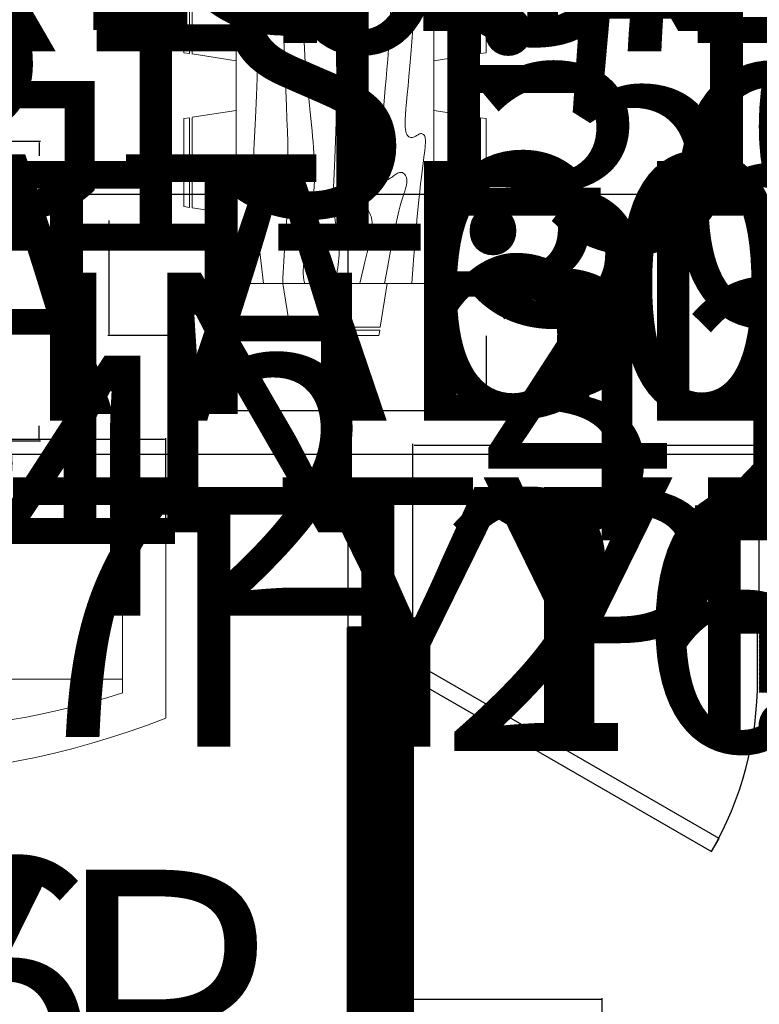
# Model space of a CAD drawing. Units: inches. Extents: x 1173 to 2157, y 515 to 1129.
# Tile 5 of 13: x 1475 to 1578, y 743 to 880. Entities that reach past the tile are written whole.
import ezdxf

# ---------------------------------------------------------------- set-up
doc = ezdxf.new("R2010")
doc.units = ezdxf.units.IN
doc.header["$MEASUREMENT"] = 0
for name, color, linetype, lineweight in [('A-ANNO-DIMS', 2, 'Continuous', 18), ('A-DOOR', 3, 'Continuous', 25), ('A-FURN', 8, 'Continuous', 18), ('A-WALL', 7, 'Continuous', 50)]:
    doc.layers.add(name, color=color, linetype=linetype, lineweight=lineweight)
doc.layers.add('A-WALL-PATT', color=22, linetype='Continuous', lineweight=13, true_color=0xca4b0c)
doc.styles.get("Standard").update_dxf_attribs({"font": 'arial.ttf'})
doc.dimstyles.get("Standard").update_dxf_attribs({"dimtxt": 36, "dimasz": 0.18, "dimexe": 0.18, "dimexo": 0.0625, "dimgap": 0.09, "dimtad": 0, "dimtih": 1, "dimtoh": 1, "dimdec": 0, "dimrnd": 72, "dimzin": 0, "dimdsep": 46, "dimlunit": 3, "dimtxsty": 'Standard', "dimcen": 2, "dimadec": 0, "dimazin": 0, "dimtfac": 1, "dimtdec": 0, "dimtofl": 0, "dimtmove": 0, "dimatfit": 3, "dimfxl": 1, "dimtolj": 1, "dimtzin": 0, "dimarcsym": 0})

# ---------------------------------------------------------------- blocks, each defined once
blk = doc.blocks.new('*U4')
for p, q in [((0, 0), (0, 6)), ((40, 0), (40, 6))]:
    blk.add_line(p, q)
blk.add_lwpolyline([(0, 0), (34.64, -20), (35.52, -18.48), (0.87, 1.52)], close=True)
blk.add_arc((0, 0), 40, 330, 0)
blk = doc.blocks.new('Dining Set - 36 x 72 in.')
for p, q in [((-22, 27.5), (-22.1562, 26.50042)), ((-22, 27.5), (-6, 27.5)), ((-5.8437, 26.49966), (-6, 27.5)), ((6, 27.5), (5.8438, 26.50042)), ((6, 27.5), (22, 27.5)), ((22.1563, 26.49966), (22, 27.5)), ((-22.2343, 26.00059), (-23.4847, 17.99762)), ((-22.2304, 26), (-5.7608, 26)), ((-5.8416, 26.5), (-22.1534, 26.5)), ((-4.5152, 17.99762), (-5.7655, 25.99926)), ((5.7657, 26.00059), (4.5153, 17.99762)), ((5.7696, 26), (22.2392, 26)), ((22.1584, 26.5), (5.8466, 26.5)), ((23.4848, 17.99762), (22.2345, 25.99926)), ((36, 18), (-36, 18)), ((-36, 18), (-36, -18)), ((36, -18), (36, 18)), ((-44.0006, 8.23428), (-35.9976, 9.48474)), ((44.0006, 8.23428), (35.9976, 9.48474)), ((-45.5, 8), (-44.5004, 8.15617)), ((-45.5, 8), (-45.5, -8)), ((-44.5, -8.15843), (-44.5, 8.15338)), ((-44, 8.23041), (-44, -8.23915)), ((44, 8.23041), (44, -8.23915)), ((44.5, -8.15843), (44.5, 8.15338)), ((45.5, 8), (44.5005, 8.15617)), ((45.5, 8), (45.5, -8)), ((-44.4997, -8.15631), (-45.5, -8)), ((-35.9976, -9.48476), (-43.9993, -8.2345)), ((35.9976, -9.48476), (43.9993, -8.2345)), ((44.4997, -8.15631), (45.5, -8)), ((-36, -18), (36, -18)), ((-22.2343, -26.0006), (-23.4847, -17.99762)), ((-4.5152, -17.99762), (-5.7655, -25.99928)), ((5.7657, -26.0006), (4.5153, -17.99762)), ((23.4848, -17.99762), (22.2345, -25.99928)), ((-22.2304, -26), (-5.7608, -26)), ((-22, -27.5), (-22.1562, -26.50044)), ((-5.8416, -26.5), (-22.1534, -26.5)), ((-5.8437, -26.49967), (-6, -27.5)), ((5.7696, -26), (22.2392, -26)), ((6, -27.5), (5.8438, -26.50044)), ((22.1584, -26.5), (5.8466, -26.5)), ((22.1563, -26.49967), (22, -27.5)), ((-22, -27.5), (-6, -27.5)), ((6, -27.5), (22, -27.5))]:
    blk.add_line(p, q)
for points in [[(-36, 15), (-31.1772, 14.97754), (-26.8079, 14.91406), (-22.8538, 14.81543), (-19.276, 14.6875), (-16.0362, 14.53613), (-13.0957, 14.36718), (-10.4159, 14.18652), (-7.9583, 14), (-5.6904, 13.81315), (-3.6035, 13.63021), (-1.6954, 13.45508), (0.0365, 13.29166), (1.5945, 13.14388), (2.9811, 13.01562), (4.1988, 12.9108), (5.25, 12.83333), (6.1393, 12.78613), (6.8802, 12.76823), (7.4883, 12.77767), (7.9792, 12.8125), (8.3685, 12.87077), (8.6719, 12.95052), (8.9049, 13.0498), (9.0833, 13.16666), (9.2205, 13.29899), (9.3216, 13.44401), (9.3895, 13.59879), (9.4271, 13.76041), (9.4373, 13.92594), (9.4232, 14.09245), (9.3875, 14.257), (9.3333, 14.41666), (9.2638, 14.56917), (9.1836, 14.71484), (9.0975, 14.85465), (9.0104, 14.98958), (8.9272, 15.1206), (8.8529, 15.2487), (8.7922, 15.37483), (8.75, 15.5), (8.7305, 15.62467), (8.7344, 15.74739), (8.7617, 15.86621), (8.8125, 15.97916), (8.8867, 16.08431), (8.9844, 16.17968), (9.1055, 16.26334), (9.25, 16.33333), (9.4189, 16.38802), (9.6172, 16.42708), (9.8506, 16.45052), (10.125, 16.45833), (10.4463, 16.45052), (10.8203, 16.42708), (11.2529, 16.38802), (11.75, 16.33333), (12.3184, 16.26318), (12.9694, 16.17838), (13.7151, 16.07991), (14.5677, 15.96875), (15.5395, 15.84586), (16.6426, 15.71224), (17.8893, 15.56884), (19.2917, 15.41666), (20.859, 15.25667), (22.5879, 15.08984), (24.4721, 14.91715), (26.5052, 14.73958), (28.6809, 14.5581), (30.9929, 14.3737), (33.4347, 14.18733), (36, 14)], [(-36, 10), (-28.9766, 10.14274), (-23.1725, 10.20442), (-18.4241, 10.19775), (-14.5677, 10.13541), (-11.4399, 10.03011), (-8.877, 9.89453), (-6.7154, 9.74137), (-4.7917, 9.58333), (-2.9698, 9.43082), (-1.2246, 9.28515), (0.4415, 9.14534), (2.026, 9.01041), (3.5266, 8.87939), (4.9408, 8.7513), (6.266, 8.62516), (7.5, 8.5), (8.6411, 8.37549), (9.6914, 8.2539), (10.6538, 8.13818), (11.5312, 8.03125), (12.3267, 7.93603), (13.043, 7.85547), (13.6831, 7.79248), (14.25, 7.75), (14.7471, 7.7303), (15.1797, 7.73307), (15.5537, 7.75732), (15.875, 7.80208), (16.1494, 7.86637), (16.3828, 7.94922), (16.5811, 8.04964), (16.75, 8.16666), (16.8944, 8.29915), (17.0143, 8.44531), (17.1089, 8.60319), (17.1771, 8.77083), (17.218, 8.94629), (17.2305, 9.1276), (17.2137, 9.31282), (17.1667, 9.5), (17.0895, 9.6875), (16.987, 9.875), (16.8649, 10.0625), (16.7292, 10.25), (16.5856, 10.4375), (16.4401, 10.625), (16.2985, 10.8125), (16.1667, 11), (16.05, 11.18733), (15.9518, 11.3737), (15.8752, 11.5581), (15.8229, 11.73958), (15.798, 11.91715), (15.8034, 12.08984), (15.842, 12.25667), (15.9167, 12.41666), (16.0295, 12.56836), (16.1784, 12.70833), (16.3605, 12.83268), (16.5729, 12.9375), (16.8127, 13.01888), (17.0768, 13.07291), (17.3625, 13.0957), (17.6667, 13.08333), (17.9894, 13.03312), (18.3418, 12.94726), (18.7382, 12.82918), (19.1927, 12.68229), (19.7195, 12.51001), (20.3327, 12.31575), (21.0465, 12.10294), (21.875, 11.875), (22.8357, 11.63354), (23.959, 11.37304), (25.2786, 11.08618), (26.8282, 10.76562), (28.6414, 10.40405), (30.752, 9.99414), (33.1936, 9.52856), (36, 9)], [(-36, 5.5), (-30.7157, 5.3348), (-26.069, 5.20963), (-21.9946, 5.11767), (-18.4271, 5.05208), (-15.3009, 5.00602), (-12.5508, 4.97265), (-10.1112, 4.94515), (-7.9167, 4.91666), (-5.909, 4.88167), (-4.0586, 4.83984), (-2.3429, 4.79215), (-0.7396, 4.73958), (0.7739, 4.6831), (2.22, 4.6237), (3.6213, 4.56233), (5, 4.5), (6.373, 4.43782), (7.7344, 4.3776), (9.0723, 4.32129), (10.375, 4.27083), (11.6309, 4.22819), (12.8281, 4.19531), (13.9551, 4.17415), (15, 4.16666), (15.954, 4.17448), (16.819, 4.19791), (17.6001, 4.23698), (18.3021, 4.29166), (18.9299, 4.36198), (19.4883, 4.44791), (19.9823, 4.54948), (20.4167, 4.66666), (20.7969, 4.79899), (21.1302, 4.94401), (21.4245, 5.09879), (21.6875, 5.26041), (21.9271, 5.42594), (22.1511, 5.59245), (22.3672, 5.757), (22.5834, 5.91666), (22.8065, 6.06868), (23.0404, 6.21093), (23.2879, 6.34147), (23.5521, 6.45833), (23.8358, 6.55957), (24.142, 6.64323), (24.4735, 6.70735), (24.8334, 6.75), (25.2235, 6.76969), (25.642, 6.76692), (26.0858, 6.74267), (26.5521, 6.69791), (27.0379, 6.63362), (27.5404, 6.55078), (28.0565, 6.45036), (28.5834, 6.33333), (29.1242, 6.19987), (29.7071, 6.04687), (30.3661, 5.87044), (31.1354, 5.66666), (32.0493, 5.43164), (33.142, 5.16146), (34.4475, 4.85221), (36, 4.5)], [(-36, -1), (-30.7915, -0.6591), (-26.0195, -0.38216), (-21.6519, -0.16284), (-17.6563, 0.00521), (-14.0005, 0.12833), (-10.6523, 0.21289), (-7.5796, 0.26522), (-4.75, 0.29166), (-2.134, 0.29793), (0.2878, 0.28711), (2.5317, 0.26163), (4.6146, 0.22396), (6.5529, 0.17651), (8.3633, 0.12174), (10.0623, 0.06209), (11.6667, 0), (13.1899, -0.06201), (14.6341, -0.1211), (15.9982, -0.17432), (17.2813, -0.21875), (18.4823, -0.25147), (19.6003, -0.26953), (20.6343, -0.27002), (21.5834, -0.25), (22.4481, -0.20768), (23.2357, -0.14584), (23.9549, -0.06836), (24.6146, 0.02083), (25.2235, 0.11784), (25.7904, 0.21875), (26.3241, 0.31966), (26.8334, 0.41666), (27.3265, 0.50618), (27.8099, 0.58593), (28.2894, 0.65397), (28.7709, 0.70833), (29.2601, 0.74707), (29.763, 0.76823), (30.2855, 0.76985), (30.8334, 0.75), (31.4088, 0.70784), (31.9994, 0.64713), (32.589, 0.57275), (33.1615, 0.48958), (33.7008, 0.4025), (34.1908, 0.3164), (34.6153, 0.23616), (34.9584, 0.16666), (35.2099, 0.11165), (35.3848, 0.07031), (35.504, 0.04069), (35.5886, 0.02083), (35.6594, 0.00879), (35.7377, 0.0026), (35.8442, 0.00032), (36, 0)], [(-36, -6.5), (-27.1843, -6.31267), (-20.084, -6.1263), (-14.469, -5.9419), (-10.1094, -5.76042), (-6.7752, -5.58285), (-4.2363, -5.41016), (-2.2629, -5.24333), (-0.625, -5.08334), (0.8708, -4.93099), (2.2715, -4.78646), (3.5872, -4.64974), (4.8281, -4.52084), (6.0046, -4.39974), (7.127, -4.28646), (8.2053, -4.18099), (9.25, -4.08334), (10.2705, -3.99382), (11.2734, -3.91407), (12.2647, -3.84603), (13.25, -3.79167), (14.2354, -3.75293), (15.2266, -3.73177), (16.2295, -3.73015), (17.25, -3.75), (18.2912, -3.79248), (19.3451, -3.85547), (20.4009, -3.93604), (21.4479, -4.03125), (22.4754, -4.13819), (23.4727, -4.25391), (24.4289, -4.37549), (25.3334, -4.5), (26.1785, -4.62492), (26.9694, -4.74935), (27.7145, -4.87281), (28.4219, -4.99479), (29.1, -5.11483), (29.7572, -5.23242), (30.4016, -5.34709), (31.0417, -5.45834), (31.6837, -5.56437), (32.3262, -5.65821), (32.9658, -5.73153), (33.599, -5.77604), (34.2224, -5.78345), (34.8327, -5.74545), (35.4264, -5.65373), (36, -5.5)], [(-36, -10), (-26.4022, -9.81299), (-18.4675, -9.62891), (-11.9839, -9.45069), (-6.7396, -9.28125), (-2.5226, -9.12354), (0.8789, -8.98047), (3.6769, -8.85498), (6.0833, -8.75), (8.2767, -8.66765), (10.3021, -8.60677), (12.1712, -8.56543), (13.8958, -8.54167), (15.4876, -8.53353), (16.9583, -8.53907), (18.3197, -8.55632), (19.5834, -8.58334), (20.7616, -8.61841), (21.8685, -8.66081), (22.9188, -8.71004), (23.9271, -8.76563), (24.9081, -8.82707), (25.8763, -8.89388), (26.8465, -8.96558), (27.8334, -9.04167), (28.8474, -9.12118), (29.8828, -9.20117), (30.93, -9.27824), (31.9792, -9.34896), (33.0205, -9.40991), (34.0443, -9.45768), (35.0407, -9.48885), (36, -9.5)], [(-36, -14.5), (-30.0881, -14.33513), (-25.0332, -14.21224), (-20.7312, -14.12647), (-17.0781, -14.07292), (-13.97, -14.04671), (-11.3027, -14.04297), (-8.9724, -14.05681), (-6.875, -14.08334), (-4.9224, -14.11833), (-3.0905, -14.16016), (-1.3709, -14.20785), (0.2448, -14.26042), (1.7647, -14.3169), (3.1973, -14.3763), (4.5507, -14.43767), (5.8333, -14.5), (7.0554, -14.5621), (8.235, -14.62175), (9.3922, -14.67652), (10.5469, -14.72396), (11.7192, -14.76164), (12.929, -14.78711), (14.1965, -14.79794), (15.5417, -14.79167), (16.9933, -14.76424), (18.6152, -14.70508), (20.4804, -14.60197), (22.6615, -14.44271), (25.2312, -14.21509), (28.2624, -13.9069), (31.8277, -13.50594), (36, -13)]]:
    blk.add_lwpolyline(points)
blk = doc.blocks.new('Sofa - Roundback 7 ft.')
for p, q in [((-12.00002, -32.4421), (-12.00003, -6.5971)), ((11.99997, -32.4421), (11.99998, -6.5971)), ((-36.000027, -34), (-36.000027, -11.4696)), ((35.99998, -34), (35.99998, -11.4696)), ((-35.999844, -13.3819), (35.9998, -13.3819)), ((-36.000027, -32.4421), (35.99998, -32.4421))]:
    blk.add_line(p, q)
for points in [[(-36.000027, -34), (-42.000027, -34), (-42.000027, -8)], [(41.99998, -8), (41.99998, -34), (35.99998, -34)]]:
    blk.add_lwpolyline(points)
for centre, radius, start, end in [((0, -114.25), 114.25, 68.43141, 111.5686), ((-0.00001, -127.1968), 121.1968, 72.72033, 107.2797)]:
    blk.add_arc(centre, radius, start, end)
blk = doc.blocks.new('*D26')
at = {"layer": 'A-ANNO-DIMS', "color": 0, "lineweight": -2, "transparency": 16777216}
for p, q in [((1577.15, 654.34), (1577.15, 661.66)), ((1577.33, 661.48), (1624.97, 661.48)), ((1625.15, 654.34), (1625.15, 661.66)), ((1625.15, 661.48), (1625.33, 661.48))]:
    blk.add_line(p, q, dxfattribs=at)
at = {"layer": 'A-ANNO-DIMS', "color": 0, "transparency": 16777216}
for points in [[(1577.33, 661.51), (1577.33, 661.45), (1577.15, 661.48)], [(1624.97, 661.51), (1624.97, 661.45), (1625.15, 661.48)]]:
    blk.add_solid(points, dxfattribs=at)
at = {"layer": 'Defpoints', "color": 0, "transparency": 16777216}
for p in [(1625.15, 661.48), (1577.15, 654.28), (1625.15, 654.28)]:
    blk.add_point(p, dxfattribs=at)
at = {"layer": 'A-ANNO-DIMS', "color": 0, "transparency": 16777216, "insert": (1831.09, 661.48), "char_height": 36, "attachment_point": 5}
blk.add_mtext('\\A1;WINDOW 48 TYP.', dxfattribs=at)
blk = doc.blocks.new('*D30')
at = {"layer": 'A-ANNO-DIMS', "color": 0, "lineweight": -2, "transparency": 16777216}
for p, q in [((1555.97, 736.03), (1563.78, 736.03)), ((1563.6, 735.85), (1563.6, 729.12)), ((1563.6, 684.97), (1563.6, 691.71)), ((1555.97, 684.79), (1563.78, 684.79))]:
    blk.add_line(p, q, dxfattribs=at)
at = {"layer": 'A-ANNO-DIMS', "color": 0, "transparency": 16777216}
for points in [[(1563.57, 735.85), (1563.63, 735.85), (1563.6, 736.03)], [(1563.57, 684.97), (1563.63, 684.97), (1563.6, 684.79)]]:
    blk.add_solid(points, dxfattribs=at)
at = {"layer": 'Defpoints', "color": 0, "transparency": 16777216}
for p in [(1555.91, 736.03), (1563.6, 736.03), (1555.91, 684.79)]:
    blk.add_point(p, dxfattribs=at)
at = {"layer": 'A-ANNO-DIMS', "color": 0, "transparency": 16777216, "insert": (1563.6, 710.41), "char_height": 36, "attachment_point": 5}
blk.add_mtext('\\A1;DESK 51 TYP.', dxfattribs=at)
blk = doc.blocks.new('*D31')
at = {"layer": 'A-ANNO-DIMS', "color": 0, "lineweight": -2, "transparency": 16777216}
for p, q in [((1529.44, 743.72), (1529.26, 743.72)), ((1529.44, 736.09), (1529.44, 743.9)), ((1555.73, 743.72), (1529.62, 743.72)), ((1555.91, 736.09), (1555.91, 743.9))]:
    blk.add_line(p, q, dxfattribs=at)
at = {"layer": 'A-ANNO-DIMS', "color": 0, "transparency": 16777216}
for points in [[(1529.62, 743.75), (1529.62, 743.69), (1529.44, 743.72)], [(1555.73, 743.75), (1555.73, 743.69), (1555.91, 743.72)]]:
    blk.add_solid(points, dxfattribs=at)
at = {"layer": 'Defpoints', "color": 0, "transparency": 16777216}
for p in [(1529.44, 743.72), (1529.44, 736.03), (1555.91, 736.03)]:
    blk.add_point(p, dxfattribs=at)
at = {"layer": 'A-ANNO-DIMS', "color": 0, "transparency": 16777216, "insert": (1441.24, 743.72), "char_height": 36, "attachment_point": 5}
blk.add_mtext('\\A1;26 TYP.', dxfattribs=at)
blk = doc.blocks.new('*D36')
at = {"layer": 'A-ANNO-DIMS', "color": 0, "lineweight": -2, "transparency": 16777216}
for p, q in [((1497.87, 905.02), (1487.37, 905.02)), ((1487.55, 904.84), (1487.55, 889.09)), ((1487.55, 835.93), (1487.55, 851.68)), ((1497.87, 835.75), (1487.37, 835.75))]:
    blk.add_line(p, q, dxfattribs=at)
at = {"layer": 'A-ANNO-DIMS', "color": 0, "transparency": 16777216}
for points in [[(1487.52, 904.84), (1487.58, 904.84), (1487.55, 905.02)], [(1487.52, 835.93), (1487.58, 835.93), (1487.55, 835.75)]]:
    blk.add_solid(points, dxfattribs=at)
at = {"layer": 'Defpoints', "color": 0, "transparency": 16777216}
for p in [(1497.94, 905.02), (1487.55, 835.75), (1497.94, 835.75)]:
    blk.add_point(p, dxfattribs=at)
at = {"layer": 'A-ANNO-DIMS', "color": 0, "transparency": 16777216, "insert": (1487.55, 870.38), "char_height": 36, "attachment_point": 5}
blk.add_mtext('\\A1;DINING SET 69', dxfattribs=at)
blk = doc.blocks.new('*D37')
at = {"layer": 'A-ANNO-DIMS', "color": 0, "lineweight": -2, "transparency": 16777216}
for p, q in [((1497.94, 835.69), (1497.94, 825.18)), ((1539.8, 835.69), (1539.8, 825.18)), ((1498.12, 825.36), (1539.62, 825.36)), ((1539.8, 825.36), (1539.98, 825.36))]:
    blk.add_line(p, q, dxfattribs=at)
at = {"layer": 'A-ANNO-DIMS', "color": 0, "transparency": 16777216}
for points in [[(1498.12, 825.39), (1498.12, 825.33), (1497.94, 825.36)], [(1539.62, 825.39), (1539.62, 825.33), (1539.8, 825.36)]]:
    blk.add_solid(points, dxfattribs=at)
at = {"layer": 'Defpoints', "color": 0, "transparency": 16777216}
for p in [(1497.94, 835.75), (1539.8, 835.75), (1539.8, 825.36)]:
    blk.add_point(p, dxfattribs=at)
at = {"layer": 'A-ANNO-DIMS', "color": 0, "transparency": 16777216, "insert": (1566.4, 825.36), "char_height": 36, "attachment_point": 5}
blk.add_mtext('\\A1;42', dxfattribs=at)
blk = doc.blocks.new('*D38')
at = {"layer": 'A-ANNO-DIMS', "color": 0, "lineweight": -2, "transparency": 16777216}
for p, q in [((1471.69, 862.7), (1478.04, 862.7)), ((1477.86, 862.52), (1477.86, 860.65)), ((1477.86, 821.35), (1477.86, 823.22)), ((1471.69, 821.17), (1478.04, 821.17))]:
    blk.add_line(p, q, dxfattribs=at)
at = {"layer": 'A-ANNO-DIMS', "color": 0, "transparency": 16777216}
for points in [[(1477.83, 862.52), (1477.89, 862.52), (1477.86, 862.7)], [(1477.83, 821.35), (1477.89, 821.35), (1477.86, 821.17)]]:
    blk.add_solid(points, dxfattribs=at)
at = {"layer": 'Defpoints', "color": 0, "transparency": 16777216}
for p in [(1471.63, 862.7), (1477.86, 862.7), (1471.63, 821.17)]:
    blk.add_point(p, dxfattribs=at)
at = {"layer": 'A-ANNO-DIMS', "color": 0, "transparency": 16777216, "insert": (1477.86, 841.93), "char_height": 36, "attachment_point": 5}
blk.add_mtext('\\A1;COFFEE TABLE 42', dxfattribs=at)
blk = doc.blocks.new('*D39')
at = {"layer": 'A-ANNO-DIMS', "color": 0, "lineweight": -2, "transparency": 16777216}
for p, q in [((1430.11, 821.11), (1430.11, 814.76)), ((1471.63, 821.11), (1471.63, 814.76)), ((1430.29, 814.94), (1471.45, 814.94)), ((1471.63, 814.94), (1471.81, 814.94))]:
    blk.add_line(p, q, dxfattribs=at)
at = {"layer": 'A-ANNO-DIMS', "color": 0, "transparency": 16777216}
for points in [[(1430.29, 814.97), (1430.29, 814.91), (1430.11, 814.94)], [(1471.45, 814.97), (1471.45, 814.91), (1471.63, 814.94)]]:
    blk.add_solid(points, dxfattribs=at)
at = {"layer": 'Defpoints', "color": 0, "transparency": 16777216}
for p in [(1430.11, 821.17), (1471.63, 821.17), (1471.63, 814.94)]:
    blk.add_point(p, dxfattribs=at)
at = {"layer": 'A-ANNO-DIMS', "color": 0, "transparency": 16777216, "insert": (1498.22, 814.94), "char_height": 36, "attachment_point": 5}
blk.add_mtext('\\A1;42', dxfattribs=at)
blk = doc.blocks.new('*D40')
at = {"layer": 'A-ANNO-DIMS', "color": 0, "lineweight": -2, "transparency": 16777216}
for p, q in [((1422.73, 872.86), (1431.84, 872.86)), ((1431.66, 872.68), (1431.66, 861.58)), ((1431.66, 813.04), (1431.66, 824.15)), ((1422.73, 812.86), (1431.84, 812.86))]:
    blk.add_line(p, q, dxfattribs=at)
at = {"layer": 'A-ANNO-DIMS', "color": 0, "transparency": 16777216}
for points in [[(1431.63, 872.68), (1431.69, 872.68), (1431.66, 872.86)], [(1431.63, 813.04), (1431.69, 813.04), (1431.66, 812.86)]]:
    blk.add_solid(points, dxfattribs=at)
at = {"layer": 'Defpoints', "color": 0, "transparency": 16777216}
for p in [(1422.66, 872.86), (1431.66, 872.86), (1422.66, 812.86)]:
    blk.add_point(p, dxfattribs=at)
at = {"layer": 'A-ANNO-DIMS', "color": 0, "transparency": 16777216, "insert": (1431.66, 842.86), "char_height": 36, "attachment_point": 5}
blk.add_mtext('\\A1;LOVESEAT 60', dxfattribs=at)
blk = doc.blocks.new('*D42')
at = {"layer": 'A-ANNO-DIMS', "color": 0, "lineweight": -2, "transparency": 16777216}
for p, q in [((1411.43, 808.8), (1411.43, 821.52)), ((1495.43, 808.8), (1495.43, 821.52)), ((1411.43, 821.34), (1411.25, 821.34)), ((1495.25, 821.34), (1411.61, 821.34))]:
    blk.add_line(p, q, dxfattribs=at)
at = {"layer": 'A-ANNO-DIMS', "color": 0, "transparency": 16777216}
for points in [[(1411.61, 821.37), (1411.61, 821.31), (1411.43, 821.34)], [(1495.25, 821.37), (1495.25, 821.31), (1495.43, 821.34)]]:
    blk.add_solid(points, dxfattribs=at)
at = {"layer": 'Defpoints', "color": 0, "transparency": 16777216}
for p in [(1411.43, 821.34), (1411.43, 808.74), (1495.43, 808.74)]:
    blk.add_point(p, dxfattribs=at)
at = {"layer": 'A-ANNO-DIMS', "color": 0, "transparency": 16777216, "insert": (1310.09, 821.34), "char_height": 36, "attachment_point": 5}
blk.add_mtext('\\A1;SOFA 84', dxfattribs=at)
blk = doc.blocks.new('*D46')
at = {"layer": 'A-ANNO-DIMS', "color": 0, "lineweight": -2, "transparency": 16777216}
for p, q in [((1646.37, 911.98), (1645.86, 896.32)), ((1648.72, 912.09), (1646.2, 912.17)), ((1645.85, 895.96), (1645.67, 895.96)), ((1648.2, 896.07), (1645.68, 896.15)), ((1645.86, 896.14), (1645.85, 895.96))]:
    blk.add_line(p, q, dxfattribs=at)
at = {"layer": 'A-ANNO-DIMS', "color": 0, "transparency": 16777216}
for points in [[(1646.34, 911.99), (1646.4, 911.98), (1646.38, 912.16)], [(1645.83, 896.32), (1645.89, 896.32), (1645.86, 896.14)]]:
    blk.add_solid(points, dxfattribs=at)
at = {"layer": 'Defpoints', "color": 0, "transparency": 16777216}
for p in [(1648.78, 912.09), (1645.86, 896.14), (1648.26, 896.06)]:
    blk.add_point(p, dxfattribs=at)
at = {"layer": 'A-ANNO-DIMS', "color": 0, "transparency": 16777216, "insert": (1538.16, 895.96), "char_height": 36, "attachment_point": 5}
blk.add_mtext('\\A1;BASIN 16', dxfattribs=at)
blk = doc.blocks.new('*D48')
at = {"layer": 'A-ANNO-DIMS', "color": 0, "lineweight": -2, "transparency": 16777216}
for p, q in [((1592.53, 826.46), (1592.35, 826.47)), ((1592.38, 821.85), (1592.54, 826.64)), ((1623.53, 825.46), (1592.71, 826.46)), ((1623.56, 820.84), (1623.71, 825.64))]:
    blk.add_line(p, q, dxfattribs=at)
at = {"layer": 'A-ANNO-DIMS', "color": 0, "transparency": 16777216}
for points in [[(1592.71, 826.49), (1592.71, 826.43), (1592.53, 826.46)], [(1623.53, 825.49), (1623.53, 825.43), (1623.71, 825.46)]]:
    blk.add_solid(points, dxfattribs=at)
at = {"layer": 'Defpoints', "color": 0, "transparency": 16777216}
for p in [(1592.53, 826.46), (1592.38, 821.79), (1623.56, 820.78)]:
    blk.add_point(p, dxfattribs=at)
at = {"layer": 'A-ANNO-DIMS', "color": 0, "transparency": 16777216, "insert": (1488.3, 826.47), "char_height": 36, "attachment_point": 5}
blk.add_mtext('\\A1;BASIN 31', dxfattribs=at)
blk = doc.blocks.new('*D49')
at = {"layer": 'A-ANNO-DIMS', "color": 0, "lineweight": -2, "transparency": 16777216}
for p, q in [((1587.7, 821.76), (1586.89, 796.55)), ((1592.32, 821.79), (1587.52, 821.94)), ((1586.87, 796.19), (1586.69, 796.19)), ((1591.49, 796.22), (1586.7, 796.37)), ((1586.88, 796.37), (1586.87, 796.19))]:
    blk.add_line(p, q, dxfattribs=at)
at = {"layer": 'A-ANNO-DIMS', "color": 0, "transparency": 16777216}
for points in [[(1587.67, 821.76), (1587.73, 821.76), (1587.7, 821.94)], [(1586.86, 796.55), (1586.92, 796.54), (1586.88, 796.37)]]:
    blk.add_solid(points, dxfattribs=at)
at = {"layer": 'Defpoints', "color": 0, "transparency": 16777216}
for p in [(1592.38, 821.79), (1586.88, 796.37), (1591.56, 796.22)]:
    blk.add_point(p, dxfattribs=at)
at = {"layer": 'A-ANNO-DIMS', "color": 0, "transparency": 16777216, "insert": (1560.52, 796.19), "char_height": 36, "attachment_point": 5}
blk.add_mtext('\\A1;26', dxfattribs=at)
blk = doc.blocks.new('*D50')
at = {"layer": 'A-ANNO-DIMS', "color": 0, "lineweight": -2, "transparency": 16777216}
for p, q in [((1603.33, 798.21), (1603.33, 796.59)), ((1613.33, 798.21), (1613.33, 796.59)), ((1603.33, 796.77), (1603.15, 796.77)), ((1613.15, 796.77), (1603.51, 796.77))]:
    blk.add_line(p, q, dxfattribs=at)
at = {"layer": 'A-ANNO-DIMS', "color": 0, "transparency": 16777216}
for points in [[(1603.51, 796.8), (1603.51, 796.74), (1603.33, 796.77)], [(1613.15, 796.8), (1613.15, 796.74), (1613.33, 796.77)]]:
    blk.add_solid(points, dxfattribs=at)
at = {"layer": 'Defpoints', "color": 0, "transparency": 16777216}
for p in [(1603.33, 798.27), (1613.33, 798.27), (1603.33, 796.77)]:
    blk.add_point(p, dxfattribs=at)
at = {"layer": 'A-ANNO-DIMS', "color": 0, "transparency": 16777216, "insert": (1377.9, 796.77), "char_height": 36, "attachment_point": 5}
blk.add_mtext('\\A1;BASIN TAP 10 TYP.', dxfattribs=at)
blk = doc.blocks.new('*D51')
at = {"layer": 'A-ANNO-DIMS', "color": 0, "lineweight": -2, "transparency": 16777216}
for p, q in [((1613.4, 804.77), (1615.01, 804.77)), ((1614.83, 804.59), (1614.83, 798.45)), ((1613.4, 798.27), (1615.01, 798.27)), ((1614.83, 798.09), (1614.65, 798.09)), ((1614.83, 798.27), (1614.83, 798.09))]:
    blk.add_line(p, q, dxfattribs=at)
at = {"layer": 'A-ANNO-DIMS', "color": 0, "transparency": 16777216}
for points in [[(1614.8, 804.59), (1614.86, 804.59), (1614.83, 804.77)], [(1614.8, 798.45), (1614.86, 798.45), (1614.83, 798.27)]]:
    blk.add_solid(points, dxfattribs=at)
at = {"layer": 'Defpoints', "color": 0, "transparency": 16777216}
for p in [(1613.33, 804.77), (1613.33, 798.27), (1614.83, 798.27)]:
    blk.add_point(p, dxfattribs=at)
at = {"layer": 'A-ANNO-DIMS', "color": 0, "transparency": 16777216, "insert": (1541.08, 798.09), "char_height": 36, "attachment_point": 5}
blk.add_mtext('\\A1;7 TYP.', dxfattribs=at)
blk = doc.blocks.new('*D52')
at = {"layer": 'A-ANNO-DIMS', "color": 0, "lineweight": -2, "transparency": 16777216}
for p, q in [((1589.6, 924.28), (1580.48, 924.28)), ((1580.66, 924.1), (1580.66, 912.75)), ((1580.66, 864.46), (1580.66, 875.81)), ((1589.6, 864.28), (1580.48, 864.28))]:
    blk.add_line(p, q, dxfattribs=at)
at = {"layer": 'A-ANNO-DIMS', "color": 0, "transparency": 16777216}
for points in [[(1580.63, 924.1), (1580.69, 924.1), (1580.66, 924.28)], [(1580.63, 864.46), (1580.69, 864.46), (1580.66, 864.28)]]:
    blk.add_solid(points, dxfattribs=at)
at = {"layer": 'Defpoints', "color": 0, "transparency": 16777216}
for p in [(1580.66, 924.28), (1589.66, 924.28), (1589.66, 864.28)]:
    blk.add_point(p, dxfattribs=at)
at = {"layer": 'A-ANNO-DIMS', "color": 0, "transparency": 16777216, "insert": (1580.66, 894.28), "char_height": 36, "attachment_point": 5}
blk.add_mtext('\\A1;TUB 60', dxfattribs=at)
blk = doc.blocks.new('*D53')
at = {"layer": 'A-ANNO-DIMS', "color": 0, "lineweight": -2, "transparency": 16777216}
for p, q in [((1589.66, 864.22), (1589.66, 855.1)), ((1625.66, 864.22), (1625.66, 855.1)), ((1589.66, 855.28), (1589.48, 855.28)), ((1625.48, 855.28), (1589.84, 855.28))]:
    blk.add_line(p, q, dxfattribs=at)
at = {"layer": 'A-ANNO-DIMS', "color": 0, "transparency": 16777216}
for points in [[(1589.84, 855.31), (1589.84, 855.25), (1589.66, 855.28)], [(1625.48, 855.31), (1625.48, 855.25), (1625.66, 855.28)]]:
    blk.add_solid(points, dxfattribs=at)
at = {"layer": 'Defpoints', "color": 0, "transparency": 16777216}
for p in [(1589.66, 864.28), (1625.66, 864.28), (1589.66, 855.28)]:
    blk.add_point(p, dxfattribs=at)
at = {"layer": 'A-ANNO-DIMS', "color": 0, "transparency": 16777216, "insert": (1563.63, 855.28), "char_height": 36, "attachment_point": 5}
blk.add_mtext('\\A1;36', dxfattribs=at)
blk = doc.blocks.new('*D69')
at = {"layer": 'A-ANNO-DIMS', "color": 0, "lineweight": -2, "transparency": 16777216}
for p, q in [((1472.66, 924.22), (1472.66, 538.8)), ((1520.66, 924.22), (1520.66, 538.8)), ((1472.84, 538.98), (1520.48, 538.98)), ((1520.66, 538.98), (1520.84, 538.98))]:
    blk.add_line(p, q, dxfattribs=at)
at = {"layer": 'A-ANNO-DIMS', "color": 0, "transparency": 16777216}
for points in [[(1472.84, 539.01), (1472.84, 538.95), (1472.66, 538.98)], [(1520.48, 539.01), (1520.48, 538.95), (1520.66, 538.98)]]:
    blk.add_solid(points, dxfattribs=at)
at = {"layer": 'Defpoints', "color": 0, "transparency": 16777216}
for p in [(1472.66, 924.28), (1520.66, 924.28), (1520.66, 538.98)]:
    blk.add_point(p, dxfattribs=at)
at = {"layer": 'A-ANNO-DIMS', "color": 0, "transparency": 16777216, "insert": (1547.48, 538.98), "char_height": 36, "attachment_point": 5}
blk.add_mtext('\\A1;48', dxfattribs=at)
blk = doc.blocks.new('*D80')
at = {"layer": 'A-ANNO-DIMS', "color": 0, "lineweight": -2, "transparency": 16777216}
for p, q in [((1363.36, 745.04), (1363.36, 745.22)), ((1363.36, 745.22), (1363.54, 745.22)), ((1388.6, 745.04), (1363.18, 745.04)), ((1363.36, 720.46), (1363.36, 744.86)), ((1388.6, 720.28), (1363.18, 720.28))]:
    blk.add_line(p, q, dxfattribs=at)
at = {"layer": 'A-ANNO-DIMS', "color": 0, "transparency": 16777216}
for points in [[(1363.33, 744.86), (1363.39, 744.86), (1363.36, 745.04)], [(1363.33, 720.46), (1363.39, 720.46), (1363.36, 720.28)]]:
    blk.add_solid(points, dxfattribs=at)
at = {"layer": 'Defpoints', "color": 0, "transparency": 16777216}
for p in [(1363.36, 745.04), (1388.66, 745.04), (1388.66, 720.28)]:
    blk.add_point(p, dxfattribs=at)
at = {"layer": 'A-ANNO-DIMS', "color": 0, "transparency": 16777216, "insert": (1424.67, 745.22), "char_height": 36, "attachment_point": 5}
blk.add_mtext('\\A1;24.76', dxfattribs=at)
blk = doc.blocks.new('*D86')
at = {"layer": 'A-ANNO-DIMS', "color": 0, "lineweight": -2, "transparency": 16777216}
for p, q in [((1529.66, 795.34), (1529.66, 820.76)), ((1529.84, 820.58), (1577.48, 820.58)), ((1577.66, 795.34), (1577.66, 820.76)), ((1577.66, 820.58), (1577.84, 820.58))]:
    blk.add_line(p, q, dxfattribs=at)
at = {"layer": 'A-ANNO-DIMS', "color": 0, "transparency": 16777216}
for points in [[(1529.84, 820.61), (1529.84, 820.55), (1529.66, 820.58)], [(1577.48, 820.61), (1577.48, 820.55), (1577.66, 820.58)]]:
    blk.add_solid(points, dxfattribs=at)
at = {"layer": 'Defpoints', "color": 0, "transparency": 16777216}
for p in [(1577.66, 820.58), (1529.66, 795.28), (1577.66, 795.28)]:
    blk.add_point(p, dxfattribs=at)
at = {"layer": 'A-ANNO-DIMS', "color": 0, "transparency": 16777216, "insert": (1604.48, 820.58), "char_height": 36, "attachment_point": 5}
blk.add_mtext('\\A1;48', dxfattribs=at)
blk = doc.blocks.new('*D87')
at = {"layer": 'A-ANNO-DIMS', "color": 0, "lineweight": -2, "transparency": 16777216}
for p, q in [((1529.66, 924.22), (1529.66, 898.8)), ((1577.66, 924.22), (1577.66, 898.8)), ((1529.66, 898.98), (1529.48, 898.98)), ((1577.48, 898.98), (1529.84, 898.98))]:
    blk.add_line(p, q, dxfattribs=at)
at = {"layer": 'A-ANNO-DIMS', "color": 0, "transparency": 16777216}
for points in [[(1529.84, 899.01), (1529.84, 898.95), (1529.66, 898.98)], [(1577.48, 899.01), (1577.48, 898.95), (1577.66, 898.98)]]:
    blk.add_solid(points, dxfattribs=at)
at = {"layer": 'Defpoints', "color": 0, "transparency": 16777216}
for p in [(1529.66, 924.28), (1577.66, 924.28), (1529.66, 898.98)]:
    blk.add_point(p, dxfattribs=at)
at = {"layer": 'A-ANNO-DIMS', "color": 0, "transparency": 16777216, "insert": (1502.85, 898.98), "char_height": 36, "attachment_point": 5}
blk.add_mtext('\\A1;48', dxfattribs=at)
blk = doc.blocks.new('*D97')
at = {"layer": 'A-ANNO-DIMS', "color": 0, "lineweight": -2, "transparency": 16777216}
for p, q in [((1580.6, 855.28), (1354.18, 855.28)), ((1354.36, 855.28), (1354.36, 855.46)), ((1354.36, 855.46), (1354.54, 855.46)), ((1354.36, 819.46), (1354.36, 855.1)), ((1580.6, 819.28), (1354.18, 819.28))]:
    blk.add_line(p, q, dxfattribs=at)
at = {"layer": 'A-ANNO-DIMS', "color": 0, "transparency": 16777216}
for points in [[(1354.33, 855.1), (1354.39, 855.1), (1354.36, 855.28)], [(1354.33, 819.46), (1354.39, 819.46), (1354.36, 819.28)]]:
    blk.add_solid(points, dxfattribs=at)
at = {"layer": 'Defpoints', "color": 0, "transparency": 16777216}
for p in [(1354.36, 855.28), (1580.66, 855.28), (1580.66, 819.28)]:
    blk.add_point(p, dxfattribs=at)
at = {"layer": 'A-ANNO-DIMS', "color": 0, "transparency": 16777216, "insert": (1380.39, 855.46), "char_height": 36, "attachment_point": 5}
blk.add_mtext('\\A1;36', dxfattribs=at)
blk = doc.blocks.new('*D108')
at = {"layer": 'A-ANNO-DIMS', "color": 0, "lineweight": -2, "transparency": 16777216}
for p, q in [((1641.43, 881.4), (1641.43, 885.4)), ((1639.43, 883.4), (1643.43, 883.4)), ((1636.72, 865.51), (1638.44, 872.04)), ((1636.54, 865.51), (1636.72, 865.51))]:
    blk.add_line(p, q, dxfattribs=at)
at = {"layer": 'A-ANNO-DIMS', "color": 0, "transparency": 16777216}
blk.add_solid([(1638.41, 872.05), (1638.47, 872.04), (1638.49, 872.22)], dxfattribs=at)
at = {"layer": 'Defpoints', "color": 0, "transparency": 16777216}
for p in [(1641.43, 883.4), (1638.49, 872.22)]:
    blk.add_point(p, dxfattribs=at)
at = {"layer": 'A-ANNO-DIMS', "color": 0, "transparency": 16777216, "insert": (1505.59, 865.51), "char_height": 36, "attachment_point": 5}
blk.add_mtext('\\A1;2X R11.564', dxfattribs=at)
blk = doc.blocks.new('*D109')
at = {"layer": 'A-ANNO-DIMS', "color": 0, "lineweight": -2, "transparency": 16777216}
for p, q in [((1638.72, 893.14), (1638.9, 893.14)), ((1638.9, 893.14), (1639.74, 886.91)), ((1641.2, 874.07), (1641.2, 878.07)), ((1639.2, 876.07), (1643.2, 876.07))]:
    blk.add_line(p, q, dxfattribs=at)
at = {"layer": 'A-ANNO-DIMS', "color": 0, "transparency": 16777216}
blk.add_solid([(1639.77, 886.92), (1639.71, 886.91), (1639.77, 886.74)], dxfattribs=at)
at = {"layer": 'Defpoints', "color": 0, "transparency": 16777216}
for p in [(1639.77, 886.74), (1641.2, 876.07)]:
    blk.add_point(p, dxfattribs=at)
at = {"layer": 'A-ANNO-DIMS', "color": 0, "transparency": 16777216, "insert": (1507.71, 893.14), "char_height": 36, "attachment_point": 5}
blk.add_mtext('\\A1;2X R10.766', dxfattribs=at)

msp = doc.modelspace()

# ---------------------------------------------------------------- hatches: boundary and pattern name
at = {"layer": 'A-WALL-PATT'}
h = msp.add_hatch(dxfattribs=at)
h.set_pattern_fill('ANSI31', color=256)
h.paths.add_polyline_path([(1388.6635, 933.2805), (1388.6635, 1044.2805), (1413.7618, 1044.2805), (1413.7618, 1053.2805), (1379.6635, 1053.2805), (1379.6635, 894.1606), (1388.6635, 894.1606), (1388.6635, 924.2805), (1472.6635, 924.2805), (1472.6635, 933.2805)])
h.paths.add_polyline_path([(1520.6635, 1044.2805), (1520.6635, 1014.7866), (1520.6635, 1005.1794), (1520.7714, 1005.1794), (1520.7714, 956.4707), (1520.6635, 924.2805), (1529.6635, 924.2805), (1529.6635, 931.4788), (1529.6635, 1044.2805), (1530.8474, 1044.2805), (1570.9543, 1044.2805), (1570.9543, 1053.2805), (1461.7618, 1053.2805), (1461.7618, 1044.2805)])
h.paths.add_polyline_path([(1618.9543, 1053.2805), (1618.9543, 1044.2805), (1661.6635, 1044.2805), (1661.6635, 1043.7367), (1661.6635, 1032.8874), (1670.6635, 1032.8874), (1670.6635, 1053.2805)])
h.paths.add_polyline_path([(1661.6635, 933.2805), (1661.6635, 927.8377), (1661.6635, 924.2805), (1661.6635, 918.9156), (1670.6635, 918.9156), (1670.6635, 984.8874), (1661.6635, 984.8874), (1661.6635, 978.3712)])
h.paths.add_polyline_path([(1670.6635, 894.9156), (1661.6635, 894.9156), (1661.6635, 890.0349), (1661.9328, 890.0349), (1661.9328, 870.079), (1661.6635, 864.2805), (1589.6635, 864.2805), (1589.6635, 924.2805), (1625.553, 924.2805, -0.02455299), (1625.3782, 927.8377), (1625.3782, 933.2805), (1577.6635, 933.2805), (1577.6635, 924.2805), (1580.6635, 924.2805), (1580.6635, 855.2805), (1586.1062, 855.2805), (1589.6635, 855.2805), (1661.6635, 855.2805), (1661.6635, 826.5597), (1670.6635, 826.5597)])
h.paths.add_polyline_path([(1670.6635, 802.5597), (1661.6635, 802.5597), (1661.6635, 795.2805), (1589.6635, 795.2805), (1589.6635, 819.17, -0.02455299), (1586.1062, 818.9952), (1580.6635, 818.9952), (1580.6635, 795.2805), (1577.6635, 795.2805), (1577.6635, 786.2805), (1661.6635, 786.2805), (1661.6635, 778.5597), (1661.6635, 742.6973), (1670.6635, 742.6973)])
h.paths.add_polyline_path([(1661.6635, 654.2805), (1625.1498, 654.2805), (1625.1498, 645.2805), (1661.3656, 645.2805), (1661.6635, 645.2805), (1661.6635, 573.2805), (1520.6635, 573.2805), (1520.6635, 564.2805), (1670.6635, 564.2805), (1670.6635, 694.6973), (1661.6635, 694.6973)])
h.paths.add_polyline_path([(1529.4367, 733.4702, -0.06854064), (1529.6635, 734.2623), (1529.6635, 795.2805), (1520.6635, 795.2805), (1520.6635, 645.2805), (1577.1498, 645.2805), (1577.1498, 654.2805), (1529.6635, 654.2805), (1529.6635, 686.5626, -0.06854064), (1529.4367, 687.3547)])
h.paths.add_polyline_path([(1379.6635, 711.2805), (1388.6635, 711.2805), (1458.7214, 711.2805), (1458.7214, 720.2805), (1410.7214, 720.2805), (1388.6635, 720.2805), (1388.6635, 745.0427), (1379.6635, 745.0427)])
h.paths.add_polyline_path([(1388.6635, 846.1606), (1379.6635, 846.1606), (1379.6635, 793.0427), (1388.6635, 793.0427)])

# ---------------------------------------------------------------- linework, layer by layer
at = {"layer": 'A-WALL'}
for p, q in [((1520.6635, 645.2805), (1520.6635, 795.2805)), ((1529.6635, 795.2805), (1520.6635, 795.2805)), ((1529.6635, 654.2805), (1529.6635, 795.2805))]:
    msp.add_line(p, q, dxfattribs=at)

# ---------------------------------------------------------------- block references
at = {"layer": 'A-DOOR', "xscale": 1.194300855349839, "yscale": 1.194300855349839, "zscale": 1.194300855349839}
msp.add_blockref('*U4', (1529.6635, 788.1147), dxfattribs=at)
at = {"layer": 'A-FURN', "xscale": 0.7611912225144155, "yscale": 0.7611912225144155, "zscale": 0.7611912225144155, "rotation": 270}
msp.add_blockref('Dining Set - 36 x 72 in.', (1518.8694, 870.3828), dxfattribs=at)
at = {"layer": 'A-FURN', "rotation": 180}
msp.add_blockref('Sofa - Roundback 7 ft.', (1453.4344, 774.7398), dxfattribs=at)

# ---------------------------------------------------------------- dimensions: what is measured, and where the dimension line sits
at = {"layer": 'A-ANNO-DIMS'}
for base, p1, p2, angle, text, picture, middle in [((1487.5464, 835.7486), (1497.9367, 905.017), (1497.9367, 835.7486), 270, 'DINING SET <>', '*D36', (1487.5464, 870.3828)), ((1645.8589, 896.1412), (1648.7786, 912.0868), (1648.2623, 896.0638), 268.15447, 'BASIN <>', '*D46', (1538.1601, 895.9613)), ((1580.6635, 924.2805), (1589.6635, 864.2805), (1589.6635, 924.2805), 90, 'TUB <>', '*D52', (1580.6635, 894.2805)), ((1477.8589, 862.6955), (1471.63, 821.1697), (1471.63, 862.6955), 90, 'COFFEE TABLE <>', '*D38', (1477.8589, 841.9326)), ((1603.3335, 796.7679), (1613.3335, 798.2679), (1603.3335, 798.2679), 180, 'BASIN TAP <> TYP.', '*D50', (1377.9039, 796.7679)), ((1431.6634, 872.8622), (1422.6634, 812.8621), (1422.6634, 872.8622), 90, 'LOVESEAT <>', '*D40', (1431.6634, 842.8622)), ((1592.531, 826.4624), (1623.5567, 820.7814), (1592.3803, 821.786), 178.15447, 'BASIN <>', '*D48', (1488.3007, 826.4682)), ((1411.4344, 821.3398), (1495.4344, 808.7398), (1411.4344, 808.7398), 180, 'SOFA <>', '*D42', (1310.0894, 821.3398)), ((1614.8335, 798.2679), (1613.3335, 804.768), (1613.3335, 798.2679), 270, '<> TYP.', '*D51', (1541.0778, 798.0879)), ((1529.4367, 743.7181), (1555.9105, 736.0322), (1529.4367, 736.0322), 180, '<> TYP.', '*D31', (1441.2418, 743.7181)), ((1563.5964, 736.0322), (1555.9105, 684.7928), (1555.9105, 736.0322), 90, 'DESK <> TYP.', '*D30', (1563.5964, 710.4125))]:
    dim = msp.add_linear_dim(base=base, p1=p1, p2=p2, angle=angle, text=text, dimstyle='Standard', override={"dimdec": 0, "dimlfac": 1, "dimrnd": 0, "dimzin": 0, "dimdsep": 46, "dimlunit": 2}, dxfattribs=at)
    dim.commit()
    dim.dimension.update_dxf_attribs({"geometry": picture, "text_midpoint": middle})
for center, mpoint, picture, middle in [((1641.2, 876.0658), (1639.765, 886.7357), '*D109', (1507.7105, 893.1376)), ((1641.4252, 883.4015), (1638.487, 872.2169), '*D108', (1505.5919, 865.5062))]:
    dim = msp.add_radius_dim(center=center, mpoint=mpoint, text='2X <>', dimstyle='Standard', override={"dimdec": 3, "dimlfac": 1, "dimrnd": 0, "dimzin": 0, "dimdsep": 46, "dimlunit": 2}, dxfattribs=at)
    dim.commit()
    dim.dimension.update_dxf_attribs({"geometry": picture, "text_midpoint": middle, "dimtype": 164})
for base, p1, p2, picture, middle in [((1520.6635, 538.978), (1472.6635, 924.2805), (1520.6635, 924.2805), '*D69', (1547.4792, 538.978)), ((1539.8022, 825.3583), (1497.9367, 835.7486), (1539.8022, 835.7486), '*D37', (1566.3969, 825.3583)), ((1577.6635, 820.583), (1529.6635, 795.2805), (1577.6635, 795.2805), '*D86', (1604.4792, 820.583)), ((1471.63, 814.9408), (1430.1061, 821.1697), (1471.63, 821.1697), '*D39', (1498.2247, 814.9408))]:
    dim = msp.add_linear_dim(base=base, p1=p1, p2=p2, dimstyle='Standard', override={"dimdec": 0, "dimlfac": 1, "dimrnd": 0, "dimzin": 0, "dimdsep": 46, "dimlunit": 2}, dxfattribs=at)
    dim.commit()
    dim.dimension.update_dxf_attribs({"geometry": picture, "text_midpoint": middle})
for base, p1, p2, angle, override, picture, middle in [((1529.6635, 898.978), (1577.6635, 924.2805), (1529.6635, 924.2805), 180, {"dimdec": 0, "dimlfac": 1, "dimrnd": 0, "dimzin": 0, "dimdsep": 46, "dimlunit": 2}, '*D87', (1502.8478, 898.978)), ((1354.361, 855.2805), (1580.6635, 819.2805), (1580.6635, 855.2805), 90, {"dimdec": 0, "dimlfac": 1, "dimrnd": 0, "dimzin": 0, "dimdsep": 46, "dimlunit": 2}, '*D97', (1380.3908, 855.4605)), ((1589.6635, 855.2805), (1625.6635, 864.2805), (1589.6635, 864.2805), 180, {"dimdec": 0, "dimlfac": 1, "dimrnd": 0, "dimzin": 0, "dimdsep": 46, "dimlunit": 2}, '*D53', (1563.6336, 855.2805)), ((1586.8799, 796.3658), (1592.3803, 821.786), (1591.5564, 796.2151), 268.15447, {"dimdec": 0, "dimlfac": 1, "dimrnd": 0, "dimzin": 0, "dimdsep": 46, "dimlunit": 2}, '*D49', (1560.525, 796.1859)), ((1363.361, 745.0427), (1388.6635, 720.2805), (1388.6635, 745.0427), 90, {"dimdec": 2, "dimlfac": 1, "dimrnd": 0, "dimzin": 0, "dimdsep": 46, "dimlunit": 2}, '*D80', (1424.6664, 745.2227))]:
    dim = msp.add_linear_dim(base=base, p1=p1, p2=p2, angle=angle, dimstyle='Standard', override=override, dxfattribs=at)
    dim.commit()
    dim.dimension.update_dxf_attribs({"geometry": picture, "text_midpoint": middle})
dim = msp.add_linear_dim(base=(1625.1498, 661.4805), p1=(1577.1498, 654.2805), p2=(1625.1498, 654.2805), text='WINDOW <> TYP.', dimstyle='Standard', override={"dimdec": 0, "dimlfac": 1, "dimrnd": 0, "dimzin": 0, "dimdsep": 46, "dimlunit": 2}, dxfattribs=at)
dim.commit()
dim.dimension.update_dxf_attribs({"geometry": '*D26', "text_midpoint": (1831.0938, 661.4805)})

doc.saveas('drawing.dxf')
